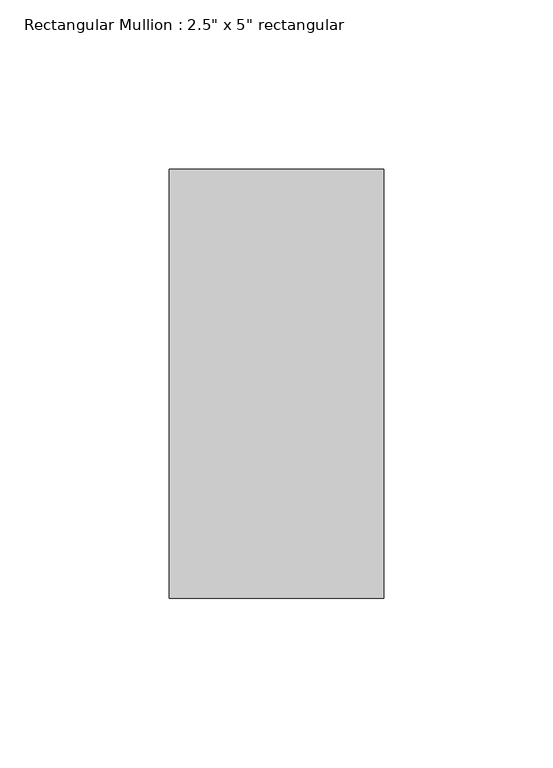
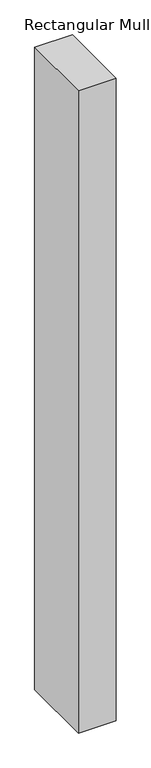
"""IFC4 building model written with IfcOpenShell, lengths in millimetres: member geometry."""

from ifc_helpers import new_model, si_unit, frame, origin, place, context, project, spatial, polyline, outline, extrude, source, transform, mapped, element, save


def member_1825c13a(model_context):
    return source(origin(), model_context, "Body", "SweptSolid", [
        extrude(outline(polyline([(0.0, 63.5), (0.0, -63.5), (-63.5, -63.5), (-63.5, 63.5), (0.0, 63.5)])), frame((0.0, 0.0, -1140.8833333), z_axis=(0.0, 0.0, 1.0), x_axis=(1.0, 0.0, 0.0)), (0.0, 0.0, 1.0), 1140.8833333),
    ])


if __name__ == "__main__":
    model = new_model("IFC4")
    model_context = context("Model", 3, world=origin())
    ifc_project = project(units=[si_unit("LENGTHUNIT", "METRE", prefix="MILLI")], contexts=[model_context])
    site = spatial("IfcSite", under=ifc_project)
    building = spatial("IfcBuilding", under=site)
    placement = place(None, origin())
    member_shape = member_1825c13a(model_context)
    element("IfcMember", 1, ObjectType="Rectangular Mullion : 2.5\" x 5\" rectangular", at=placement, inside=building, context=model_context, shape_type="MappedRepresentation", body=[
        mapped(member_shape, transform((0.0, 0.0, 0.0), x_axis=(1.0, 0.0, 0.0), y_axis=(0.0, 1.0, 0.0), z_axis=(0.0, 0.0, 1.0))),
    ])
    save(model, "model.ifc")

# Revit data of these elements
# Type "Rectangular Mullion : 2.5\" x 5\" rectangular"
#   built-in parameter 1007304 = 0.416667 (stored number, unit not read)
#   built-in parameter 1007301 = 0.104167 (stored number, unit not read)
#   built-in parameter 1007300 = 0.104167 (stored number, unit not read)
# Element 1 (IfcMember, "Rectangular Mullion : 2.5\" x 5\" rectangular")
#   Materials on its faces: "Aluminum"
# Materials
#   "Aluminum": class "Metal", colour RGB 247 247 247, transparency 0, Description = "Aluminum 6061", Cost = 0
